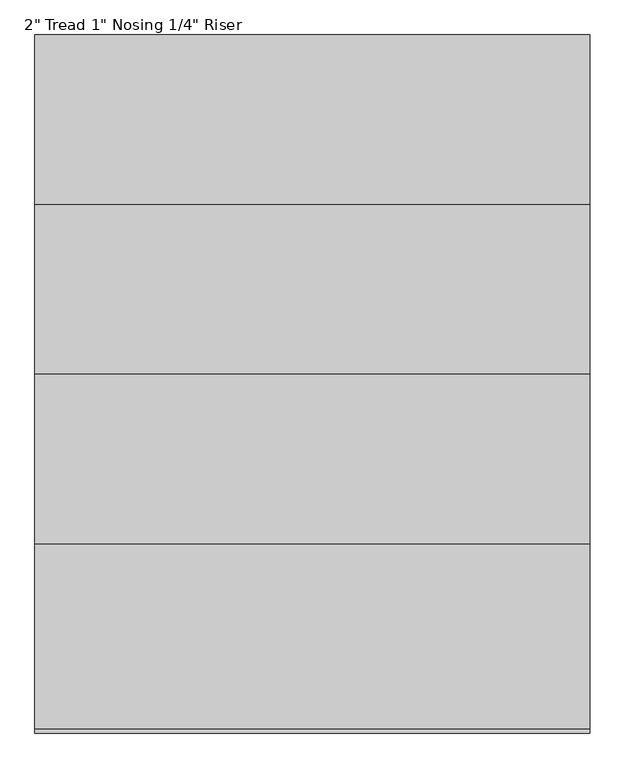
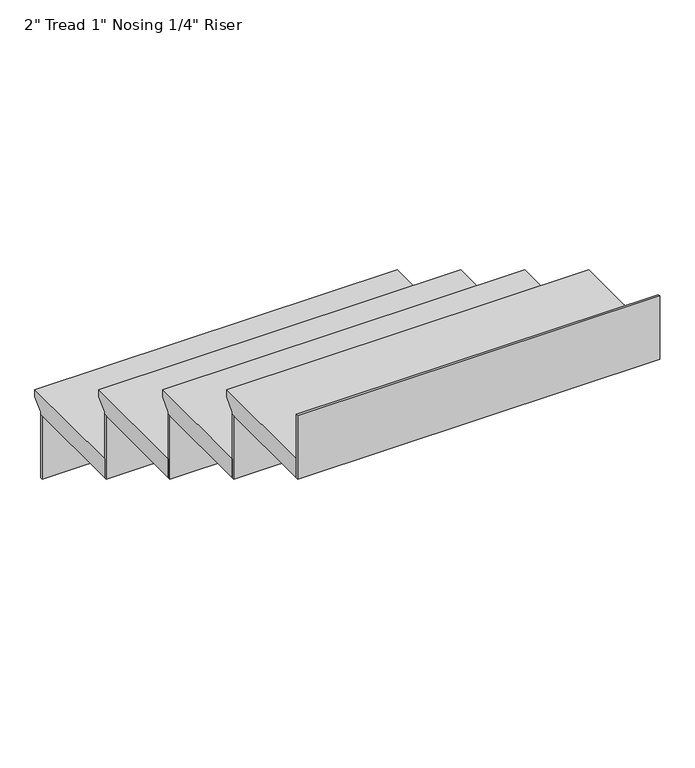
"""IFC4 building model written with IfcOpenShell, lengths in millimetres: stair flight geometry."""

from ifc_helpers import new_model, si_unit, frame, origin, place, context, project, spatial, polyline, outline, extrude, source, transform, mapped, element, save


def stair_flight_7705a6e8(model_context):
    return source(origin(), model_context, "Body", "SweptSolid", [
        extrude(outline(polyline([(22889.9216096, 39797.2839133), (23194.7216096, 39797.2839133), (23194.7216096, 39778.2339133), (23169.3216096, 39752.8339133), (23169.3216096, 39746.4839133), (22889.9216096, 39746.4839133), (22889.9216096, 39797.2839133)])), frame((-2398.2415084, 0.0, 0.0), z_axis=(1.0, 0.0, 0.0), x_axis=(0.0, 1.0, 0.0)), (0.0, 0.0, 1.0), 914.4),
        extrude(outline(polyline([(-2398.2415084, 23162.9716096), (-2398.2415084, 23169.3216096), (-1483.8415084, 23169.3216096), (-1483.8415084, 23162.9716096), (-2398.2415084, 23162.9716096)])), frame((0.0, 0.0, 39577.1505799), z_axis=(0.0, 0.0, 1.0), x_axis=(1.0, 0.0, 0.0)), (0.0, 0.0, 1.0), 169.3333333),
        extrude(outline(polyline([(-2398.2415084, 22883.5716096), (-2398.2415084, 22889.9216096), (-1483.8415084, 22889.9216096), (-1483.8415084, 22883.5716096), (-2398.2415084, 22883.5716096)])), frame((0.0, 0.0, 39746.4839133), z_axis=(0.0, 0.0, 1.0), x_axis=(1.0, 0.0, 0.0)), (0.0, 0.0, 1.0), 169.3333333),
        extrude(outline(polyline([(22610.5216096, 39966.6172466), (22915.3216096, 39966.6172466), (22915.3216096, 39947.5672466), (22889.9216096, 39922.1672466), (22889.9216096, 39915.8172466), (22610.5216096, 39915.8172466), (22610.5216096, 39966.6172466)])), frame((-2398.2415084, 0.0, 0.0), z_axis=(1.0, 0.0, 0.0), x_axis=(0.0, 1.0, 0.0)), (0.0, 0.0, 1.0), 914.4),
        extrude(outline(polyline([(-2398.2415084, 22604.1716096), (-2398.2415084, 22610.5216096), (-1483.8415084, 22610.5216096), (-1483.8415084, 22604.1716096), (-2398.2415084, 22604.1716096)])), frame((0.0, 0.0, 39915.8172466), z_axis=(0.0, 0.0, 1.0), x_axis=(1.0, 0.0, 0.0)), (0.0, 0.0, 1.0), 169.3333333),
        extrude(outline(polyline([(22331.1216096, 40135.9505799), (22635.9216096, 40135.9505799), (22635.9216096, 40116.9005799), (22610.5216096, 40091.5005799), (22610.5216096, 40085.1505799), (22331.1216096, 40085.1505799), (22331.1216096, 40135.9505799)])), frame((-2398.2415084, 0.0, 0.0), z_axis=(1.0, 0.0, 0.0), x_axis=(0.0, 1.0, 0.0)), (0.0, 0.0, 1.0), 914.4),
        extrude(outline(polyline([(-2398.2415084, 22324.7716096), (-2398.2415084, 22331.1216096), (-1483.8415084, 22331.1216096), (-1483.8415084, 22324.7716096), (-2398.2415084, 22324.7716096)])), frame((0.0, 0.0, 40085.1505799), z_axis=(0.0, 0.0, 1.0), x_axis=(1.0, 0.0, 0.0)), (0.0, 0.0, 1.0), 169.3333333),
        extrude(outline(polyline([(-2398.2415084, 22045.3716096), (-2398.2415084, 22051.7216096), (-1483.8415084, 22051.7216096), (-1483.8415084, 22045.3716096), (-2398.2415084, 22045.3716096)])), frame((0.0, 0.0, 40254.4839133), z_axis=(0.0, 0.0, 1.0), x_axis=(1.0, 0.0, 0.0)), (0.0, 0.0, 1.0), 169.3333333),
        extrude(outline(polyline([(22051.7216096, 40305.2839133), (22356.5216096, 40305.2839133), (22356.5216096, 40286.2339133), (22331.1216096, 40260.8339133), (22331.1216096, 40254.4839133), (22051.7216096, 40254.4839133), (22051.7216096, 40305.2839133)])), frame((-2398.2415084, 0.0, 0.0), z_axis=(1.0, 0.0, 0.0), x_axis=(0.0, 1.0, 0.0)), (0.0, 0.0, 1.0), 914.4),
    ])


if __name__ == "__main__":
    model = new_model("IFC4")
    model_context = context("Model", 3, world=origin())
    ifc_project = project(units=[si_unit("LENGTHUNIT", "METRE", prefix="MILLI")], contexts=[model_context])
    site = spatial("IfcSite", under=ifc_project)
    building = spatial("IfcBuilding", under=site)
    placement = place(None, origin())
    stair_flight_shape = stair_flight_7705a6e8(model_context)
    element("IfcStairFlight", 1, ObjectType="2\" Tread 1\" Nosing 1/4\" Riser", at=placement, inside=building, context=model_context, shape_type="MappedRepresentation", body=[
        mapped(stair_flight_shape, transform((0.0, 0.0, 0.0), x_axis=(1.0, 0.0, 0.0), y_axis=(0.0, 1.0, 0.0), z_axis=(0.0, 0.0, 1.0))),
    ])
    save(model, "model.ifc")
